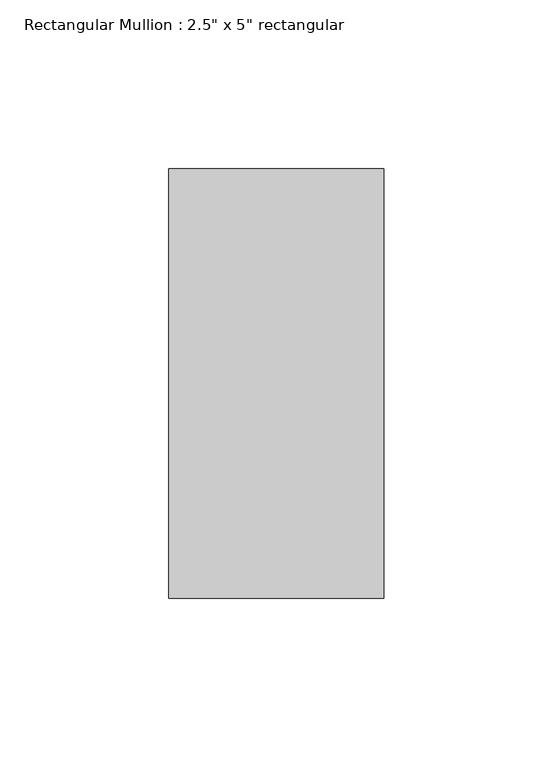
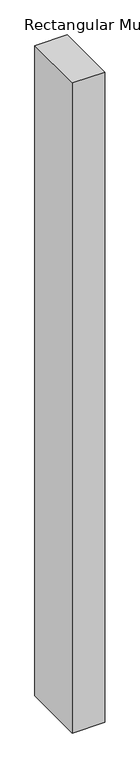
"""IFC4 building model written with IfcOpenShell, lengths in millimetres: member geometry."""

from ifc_helpers import new_model, si_unit, frame, origin, place, context, project, spatial, polyline, outline, extrude, source, transform, mapped, element, save


def member_d4123ca4(model_context):
    return source(origin(), model_context, "Body", "SweptSolid", [
        extrude(outline(polyline([(0.0, 63.5), (0.0, -63.5), (-63.5, -63.5), (-63.5, 63.5), (0.0, 63.5)])), frame((0.0, 0.0, -1347.9161516), z_axis=(0.0, 0.0, 1.0), x_axis=(1.0, 0.0, 0.0)), (0.0, 0.0, 1.0), 1347.9161516),
    ])


if __name__ == "__main__":
    model = new_model("IFC4")
    model_context = context("Model", 3, world=origin())
    ifc_project = project(units=[si_unit("LENGTHUNIT", "METRE", prefix="MILLI")], contexts=[model_context])
    site = spatial("IfcSite", under=ifc_project)
    building = spatial("IfcBuilding", under=site)
    placement = place(None, origin())
    member_shape = member_d4123ca4(model_context)
    element("IfcMember", 1, ObjectType="Rectangular Mullion : 2.5\" x 5\" rectangular", at=placement, inside=building, context=model_context, shape_type="MappedRepresentation", body=[
        mapped(member_shape, transform((0.0, 0.0, 0.0), x_axis=(1.0, 0.0, 0.0), y_axis=(0.0, 1.0, 0.0), z_axis=(0.0, 0.0, 1.0))),
    ])
    save(model, "model.ifc")

# Revit data of these elements
# Type "Rectangular Mullion : 2.5\" x 5\" rectangular"
#   built-in parameter 1007304 = 0.416667 (stored number, unit not read)
#   built-in parameter 1007301 = 0.104167 (stored number, unit not read)
#   built-in parameter 1007300 = 0.104167 (stored number, unit not read)
# Element 1 (IfcMember, "Rectangular Mullion : 2.5\" x 5\" rectangular")
#   Materials on its faces: "Aluminum"
# Materials
#   "Aluminum": class "Metal", colour RGB 247 247 247, transparency 0, Description = "Aluminum 6061", Cost = 0
